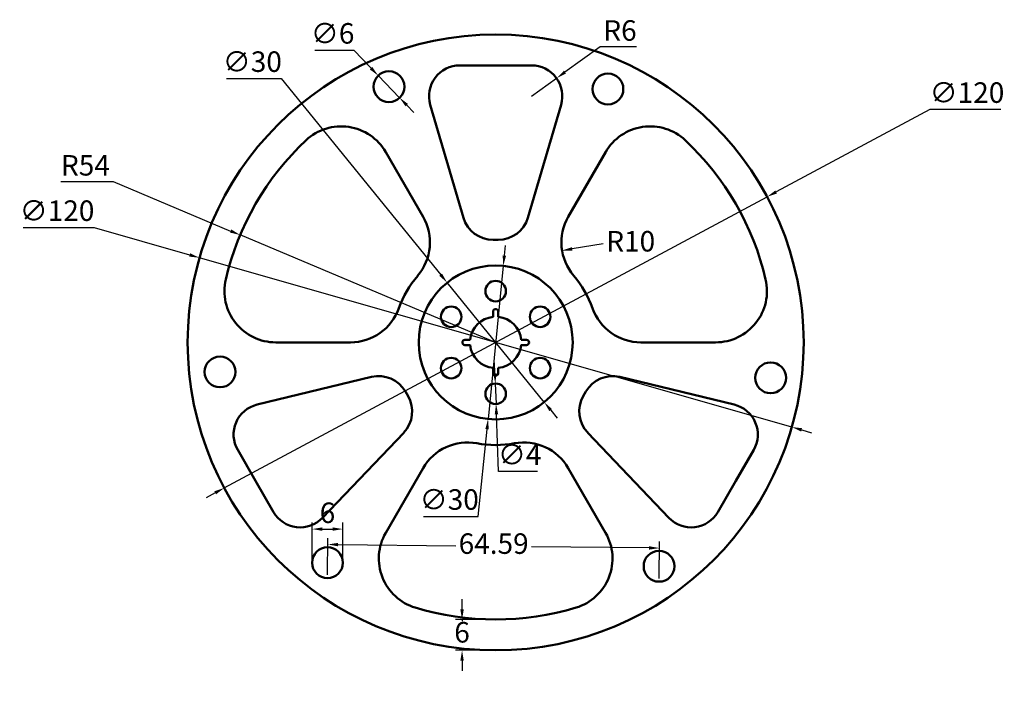
# Model space of a CAD drawing. Units: millimetres. Extents: x 45 to 237, y 22 to 152.
import ezdxf

# ---------------------------------------------------------------- set-up
doc = ezdxf.new("R2010")
doc.units = ezdxf.units.MM
doc.layers.add('M-DIMS', color=2, linetype='Continuous', lineweight=25)
doc.layers.add('M-OUTL', color=7, linetype='Continuous', lineweight=50)
doc.styles.get("Standard").update_dxf_attribs({"font": 'arial.ttf'})
doc.dimstyles.new('ISO-25', dxfattribs={"dimtxt": 4, "dimasz": 2, "dimexe": 1.25, "dimexo": 0.625, "dimtad": 1, "dimtih": 1, "dimtoh": 1, "dimtxsty": 'Standard', "dimcen": 2.5, "dimadec": 0, "dimazin": 0, "dimtfac": 1, "dimtmove": 0, "dimatfit": 3, "dimfxl": 1, "dimarcsym": 0})

# ---------------------------------------------------------------- blocks, each defined once
blk = doc.blocks.new('*U1')
for p, q in [((-0.5, 0.26), (-0.5, -0.76)), ((0.5, 0.26), (0.5, -0.76))]:
    blk.add_line(p, q)
blk.add_arc((0, 0.26), 0.5, 0, 180)
blk = doc.blocks.new('*U2')
at = {"layer": 'M-OUTL', "color": 0, "linetype": 'ByBlock', "lineweight": -2, "transparency": 16777216}
blk.add_blockref('*U1', (138.18, 94.73), dxfattribs=at)
for p, rotation in [((132.45, 88.99), 90), ((143.92, 88.99), 270), ((138.18, 83.26), 180)]:
    blk.add_blockref('*U1', p, dxfattribs=dict(at, rotation=rotation))
blk = doc.blocks.new('*U3')
blk.add_circle((0, 0), 2)
blk = doc.blocks.new('*U4')
at = {"layer": 'M-OUTL', "color": 0, "linetype": 'ByBlock', "lineweight": -2, "transparency": 16777216}
blk.add_blockref('*U3', (138.18, 98.99), dxfattribs=at)
for p, rotation in [((129.52, 93.99), 59.99999999999999), ((146.84, 93.99), 300), ((129.52, 83.99), 120), ((146.84, 83.99), 240), ((138.18, 78.99), 180)]:
    blk.add_blockref('*U3', p, dxfattribs=dict(at, rotation=rotation))
blk = doc.blocks.new('*U5')
for p, q in [((18.68, 3.44), (11.4, 16.05)), ((4.54, -21.05), (-10.02, -21.05))]:
    blk.add_line(p, q)
for centre, radius, start, end in [((2.74, 11.05), 10, 30, 133.1366), ((32.83, -21.05), 54, 133.1366, 166.8634), ((10.02, -1.56), 10, 319.4712, 30), ((-10.02, -11.05), 10, 166.8634, 270), ((32.83, -21.05), 20, 139.4712, 160.5288), ((4.54, -11.05), 10, 270, 340.5288)]:
    blk.add_arc(centre, radius, start, end)
blk = doc.blocks.new('*U6')
at = {"layer": 'M-OUTL', "color": 0, "linetype": 'ByBlock', "lineweight": -2, "transparency": 16777216}
for p, rotation in [((172.83, 106.9), 240), ((136.36, 50.04), 119.9999999999999)]:
    blk.add_blockref('*U5', p, dxfattribs=dict(at, rotation=rotation))
blk.add_blockref('*U5', (105.36, 110.05), dxfattribs=at)
blk = doc.blocks.new('*U7')
for p, q in [((0, 17), (-6.98, 17)), ((0, 17), (6.98, 17)), ((-6.27, -12.69), (-12.74, 9.31)), ((12.74, 9.31), (6.27, -12.69))]:
    blk.add_line(p, q)
for centre, start, end in [((-6.98, 11), 90, 196.3895), ((6.98, 11), 343.6105, 90), ((-0.51, -11), 196.3895, 270), ((0.51, -11), 270, 343.6105)]:
    blk.add_arc(centre, 6, start, end)
blk = doc.blocks.new('*U8')
at = {"layer": 'M-OUTL', "color": 0, "linetype": 'ByBlock', "lineweight": -2, "transparency": 16777216}
blk.add_blockref('*U7', (138.18, 125.99), dxfattribs=at)
for p, rotation in [((106.14, 70.49), 120), ((170.23, 70.49), 240)]:
    blk.add_blockref('*U7', p, dxfattribs=dict(at, rotation=rotation))
blk = doc.blocks.new('*U9')
blk.add_circle((0, 0), 3)
blk = doc.blocks.new('*U10')
at = {"layer": 'M-OUTL', "color": 0, "linetype": 'ByBlock', "lineweight": -2, "transparency": 16777216}
blk.add_blockref('*U9', (117.39, 138.83), dxfattribs=at)
for p, rotation in [((191.74, 82.09), 239.9999999999999), ((105.42, 46.07), 120)]:
    blk.add_blockref('*U9', p, dxfattribs=dict(at, rotation=rotation))
blk = doc.blocks.new('*U11')
blk.add_circle((0, 0), 3)
blk = doc.blocks.new('*U12')
at = {"layer": 'M-OUTL', "color": 0, "linetype": 'ByBlock', "lineweight": -2, "transparency": 16777216}
blk.add_blockref('*U11', (117.39, 138.83), dxfattribs=at)
for p, rotation in [((191.74, 82.09), 239.9999999999999), ((105.42, 46.07), 120)]:
    blk.add_blockref('*U11', p, dxfattribs=dict(at, rotation=rotation))
blk = doc.blocks.new('*D13')
at = {"layer": 'Defpoints', "color": 0, "transparency": 16777216}
for p in [(160.99, 108.49), (151.11, 106.9)]:
    blk.add_point(p, dxfattribs=at)
at = {"layer": 'M-DIMS', "color": 0, "lineweight": -2, "transparency": 16777216}
blk.add_line((159.09, 108.19), (153.09, 107.22), dxfattribs=at)
at = {"layer": 'M-DIMS', "color": 0, "transparency": 16777216}
blk.add_solid([(153.03, 107.55), (153.14, 106.89), (151.11, 106.9)], dxfattribs=at)
at = {"layer": 'M-DIMS', "color": 0, "transparency": 16777216, "insert": (164.49, 108.19), "char_height": 4, "attachment_point": 5}
blk.add_mtext('R10', dxfattribs=at)
blk = doc.blocks.new('*D14')
at = {"layer": 'Defpoints', "color": 0, "transparency": 16777216}
for p in [(150.04, 140.49), (145.16, 136.99)]:
    blk.add_point(p, dxfattribs=at)
at = {"layer": 'M-DIMS', "color": 0, "lineweight": -2, "transparency": 16777216}
for p, q in [((158.55, 146.59), (151.67, 141.66)), ((165.62, 146.59), (158.55, 146.59)), ((145.16, 136.99), (150.04, 140.49))]:
    blk.add_line(p, q, dxfattribs=at)
at = {"layer": 'M-DIMS', "color": 0, "transparency": 16777216}
blk.add_solid([(151.47, 141.93), (151.86, 141.39), (150.04, 140.49)], dxfattribs=at)
at = {"layer": 'M-DIMS', "color": 0, "transparency": 16777216, "insert": (162.4, 149.26), "char_height": 4, "attachment_point": 5}
blk.add_mtext('R6', dxfattribs=at)
blk = doc.blocks.new('*D15')
at = {"layer": 'Defpoints', "color": 0, "transparency": 16777216}
for p in [(115.3, 140.99), (119.47, 136.67)]:
    blk.add_point(p, dxfattribs=at)
at = {"layer": 'M-DIMS', "color": 0, "lineweight": -2, "transparency": 16777216}
for p, q in [((102.94, 145.92), (110.54, 145.92)), ((110.54, 145.92), (113.91, 142.42)), ((119.47, 136.67), (115.3, 140.99)), ((120.86, 135.23), (122.25, 133.8))]:
    blk.add_line(p, q, dxfattribs=at)
blk.add_arc((117.39, 138.83), 3, 101.9366, 157.9006, dxfattribs=at)
at = {"layer": 'M-DIMS', "color": 0, "transparency": 16777216}
for points in [[(114.15, 142.66), (113.67, 142.19), (115.3, 140.99)], [(121.1, 135.47), (120.62, 135), (119.47, 136.67)]]:
    blk.add_solid(points, dxfattribs=at)
at = {"layer": 'M-DIMS', "color": 0, "transparency": 16777216, "insert": (106.42, 148.7), "char_height": 4, "attachment_point": 5}
blk.add_mtext('∅6', dxfattribs=at)
blk = doc.blocks.new('*D16')
at = {"layer": 'Defpoints', "color": 0, "transparency": 16777216}
for p in [(88.41, 109.93), (138.18, 88.99)]:
    blk.add_point(p, dxfattribs=at)
at = {"layer": 'M-DIMS', "color": 0, "lineweight": -2, "transparency": 16777216}
for p, q in [((53.5, 120.33), (63.67, 120.33)), ((63.67, 120.33), (86.56, 110.7)), ((138.18, 88.99), (88.41, 109.93))]:
    blk.add_line(p, q, dxfattribs=at)
at = {"layer": 'M-DIMS', "color": 0, "transparency": 16777216}
blk.add_solid([(86.69, 111.01), (86.43, 110.4), (88.41, 109.93)], dxfattribs=at)
at = {"layer": 'M-DIMS', "color": 0, "transparency": 16777216, "insert": (58.27, 122.99), "char_height": 4, "attachment_point": 5}
blk.add_mtext('R54', dxfattribs=at)
blk = doc.blocks.new('*D17')
at = {"layer": 'Defpoints', "color": 0, "transparency": 16777216}
for p in [(80.5, 105.49), (195.87, 72.5)]:
    blk.add_point(p, dxfattribs=at)
at = {"layer": 'M-DIMS', "color": 0, "lineweight": -2, "transparency": 16777216}
for p, q in [((46.15, 111.37), (59.95, 111.37)), ((59.95, 111.37), (78.57, 106.04)), ((195.87, 72.5), (80.5, 105.49)), ((197.79, 71.95), (199.72, 71.4))]:
    blk.add_line(p, q, dxfattribs=at)
at = {"layer": 'M-DIMS', "color": 0, "transparency": 16777216}
for points in [[(78.66, 106.36), (78.48, 105.72), (80.5, 105.49)], [(197.89, 72.27), (197.7, 71.63), (195.87, 72.5)]]:
    blk.add_solid(points, dxfattribs=at)
at = {"layer": 'M-DIMS', "color": 0, "transparency": 16777216, "insert": (52.74, 114.15), "char_height": 4, "attachment_point": 5}
blk.add_mtext('∅120', dxfattribs=at)
blk = doc.blocks.new('*D18')
at = {"layer": 'Defpoints', "color": 0, "transparency": 16777216}
for p in [(138.11, 80.99), (138.26, 77)]:
    blk.add_point(p, dxfattribs=at)
at = {"layer": 'M-DIMS', "color": 0, "lineweight": -2, "transparency": 16777216}
for p, q in [((138.03, 82.99), (137.96, 84.99)), ((138.11, 80.99), (138.26, 77)), ((138.75, 63.84), (138.33, 75)), ((146.34, 63.84), (138.75, 63.84))]:
    blk.add_line(p, q, dxfattribs=at)
blk.add_arc((138.18, 78.99), 2, 236.3439, 1.5663, dxfattribs=at)
at = {"layer": 'M-DIMS', "color": 0, "transparency": 16777216}
for points in [[(138.37, 83), (137.7, 82.98), (138.11, 80.99)], [(138.67, 75.01), (138, 74.98), (138.26, 77)]]:
    blk.add_solid(points, dxfattribs=at)
at = {"layer": 'M-DIMS', "color": 0, "transparency": 16777216, "insert": (142.86, 66.62), "char_height": 4, "attachment_point": 5}
blk.add_mtext('∅4', dxfattribs=at)
blk = doc.blocks.new('*D19')
at = {"layer": 'Defpoints', "color": 0, "transparency": 16777216}
for p in [(128.73, 100.64), (147.64, 77.35)]:
    blk.add_point(p, dxfattribs=at)
at = {"layer": 'M-DIMS', "color": 0, "lineweight": -2, "transparency": 16777216}
for p, q in [((85.74, 140.41), (96.43, 140.41)), ((96.43, 140.41), (127.47, 102.19)), ((147.64, 77.35), (128.73, 100.64)), ((148.9, 75.8), (150.16, 74.25))]:
    blk.add_line(p, q, dxfattribs=at)
at = {"layer": 'M-DIMS', "color": 0, "transparency": 16777216}
for points in [[(127.73, 102.4), (127.21, 101.98), (128.73, 100.64)], [(149.16, 76.01), (148.64, 75.59), (147.64, 77.35)]]:
    blk.add_solid(points, dxfattribs=at)
at = {"layer": 'M-DIMS', "color": 0, "transparency": 16777216, "insert": (90.78, 143.19), "char_height": 4, "attachment_point": 5}
blk.add_mtext('∅30', dxfattribs=at)
blk = doc.blocks.new('*D20')
at = {"layer": 'Defpoints', "color": 0, "transparency": 16777216}
for p in [(139.67, 103.92), (136.7, 74.07)]:
    blk.add_point(p, dxfattribs=at)
at = {"layer": 'M-DIMS', "color": 0, "lineweight": -2, "transparency": 16777216}
for p, q in [((139.87, 105.91), (140.07, 107.9)), ((139.67, 103.92), (136.7, 74.07)), ((134.8, 55.08), (136.5, 72.08)), ((124.11, 55.08), (134.8, 55.08))]:
    blk.add_line(p, q, dxfattribs=at)
at = {"layer": 'M-DIMS', "color": 0, "transparency": 16777216}
for points in [[(139.54, 105.94), (140.2, 105.88), (139.67, 103.92)], [(136.17, 72.11), (136.83, 72.05), (136.7, 74.07)]]:
    blk.add_solid(points, dxfattribs=at)
at = {"layer": 'M-DIMS', "color": 0, "transparency": 16777216, "insert": (129.14, 57.86), "char_height": 4, "attachment_point": 5}
blk.add_mtext('∅30', dxfattribs=at)
blk = doc.blocks.new('*D21')
at = {"layer": 'Defpoints', "color": 0, "transparency": 16777216}
for p in [(108.42, 52.62), (102.42, 46.07), (108.42, 46.07)]:
    blk.add_point(p, dxfattribs=at)
at = {"layer": 'M-DIMS', "color": 0, "lineweight": -2, "transparency": 16777216}
for p, q in [((102.42, 46.69), (102.42, 53.87)), ((108.42, 46.69), (108.42, 53.87)), ((104.42, 52.62), (106.42, 52.62))]:
    blk.add_line(p, q, dxfattribs=at)
at = {"layer": 'M-DIMS', "color": 0, "transparency": 16777216}
for points in [[(104.42, 52.95), (104.42, 52.28), (102.42, 52.62)], [(106.42, 52.95), (106.42, 52.28), (108.42, 52.62)]]:
    blk.add_solid(points, dxfattribs=at)
at = {"layer": 'M-DIMS', "color": 0, "transparency": 16777216, "insert": (105.42, 55.28), "char_height": 4, "attachment_point": 5}
blk.add_mtext('6', dxfattribs=at)
blk = doc.blocks.new('*D22')
at = {"layer": 'Defpoints', "color": 0, "transparency": 16777216}
for p in [(131.63, 34.99), (138.18, 34.99), (138.18, 28.99)]:
    blk.add_point(p, dxfattribs=at)
at = {"layer": 'M-DIMS', "color": 0, "lineweight": -2, "transparency": 16777216}
for p, q in [((131.63, 36.99), (131.63, 38.99)), ((137.56, 34.99), (130.38, 34.99)), ((131.63, 34.99), (131.63, 34.66)), ((137.56, 28.99), (130.38, 28.99)), ((131.63, 28.99), (131.63, 29.33)), ((131.63, 26.99), (131.63, 24.99))]:
    blk.add_line(p, q, dxfattribs=at)
at = {"layer": 'M-DIMS', "color": 0, "transparency": 16777216}
for points in [[(131.3, 36.99), (131.97, 36.99), (131.63, 34.99)], [(131.3, 26.99), (131.97, 26.99), (131.63, 28.99)]]:
    blk.add_solid(points, dxfattribs=at)
at = {"layer": 'M-DIMS', "color": 0, "transparency": 16777216, "insert": (131.63, 31.99), "char_height": 4, "attachment_point": 5}
blk.add_mtext('6', dxfattribs=at)
blk = doc.blocks.new('*D23')
at = {"layer": 'Defpoints', "color": 0, "transparency": 16777216}
for p in [(170.08, 48.92), (105.42, 43.07), (170.01, 42.37)]:
    blk.add_point(p, dxfattribs=at)
at = {"layer": 'M-DIMS', "color": 0, "lineweight": -2, "transparency": 16777216}
for p, q in [((105.43, 43.69), (105.51, 50.87)), ((170.01, 42.99), (170.09, 50.17)), ((107.49, 49.59), (130.4, 49.35)), ((168.08, 48.94), (145.18, 49.19))]:
    blk.add_line(p, q, dxfattribs=at)
at = {"layer": 'M-DIMS', "color": 0, "transparency": 16777216}
for points in [[(107.5, 49.93), (107.49, 49.26), (105.5, 49.62)], [(168.08, 49.27), (168.07, 48.61), (170.08, 48.92)]]:
    blk.add_solid(points, dxfattribs=at)
at = {"layer": 'M-DIMS', "color": 0, "transparency": 16777216, "insert": (137.79, 49.27), "char_height": 4, "attachment_point": 5}
blk.add_mtext('64.59', dxfattribs=at)
blk = doc.blocks.new('*D24')
at = {"layer": 'Defpoints', "color": 0, "transparency": 16777216}
for p in [(191.05, 117.36), (85.31, 60.63)]:
    blk.add_point(p, dxfattribs=at)
at = {"layer": 'M-DIMS', "color": 0, "lineweight": -2, "transparency": 16777216}
for p, q in [((222.78, 134.38), (192.82, 118.31)), ((236.58, 134.38), (222.78, 134.38)), ((85.31, 60.63), (191.05, 117.36)), ((83.55, 59.68), (81.79, 58.74))]:
    blk.add_line(p, q, dxfattribs=at)
at = {"layer": 'M-DIMS', "color": 0, "transparency": 16777216}
for points in [[(192.66, 118.6), (192.97, 118.01), (191.05, 117.36)], [(83.39, 59.98), (83.71, 59.39), (85.31, 60.63)]]:
    blk.add_solid(points, dxfattribs=at)
at = {"layer": 'M-DIMS', "color": 0, "transparency": 16777216, "insert": (229.99, 137.16), "char_height": 4, "attachment_point": 5}
blk.add_mtext('∅120', dxfattribs=at)

msp = doc.modelspace()

# ---------------------------------------------------------------- linework, layer by layer
at = {"layer": 'M-OUTL'}
for p, q in [((138.183, 108.995), (137.673, 108.995)), ((138.183, 108.995), (138.694, 108.995)), ((120.608, 79.437), (121.118, 78.552)), ((155.249, 78.552), (155.759, 79.437))]:
    msp.add_line(p, q, dxfattribs=at)
for radius in [60, 15]:
    msp.add_circle((138.183, 88.995), radius, dxfattribs=at)
for start, end in [(95.73917, 174.26083), (5.73917, 84.26083), (185.73917, 264.26083), (275.73917, 354.26083)]:
    msp.add_arc((138.183, 88.995), 5, start, end, dxfattribs=at)

# ---------------------------------------------------------------- block references
at = {"layer": 'M-OUTL', "xscale": -1, "rotation": 358.7627453625808}
msp.add_blockref('*U12', (274.413, -2.963), dxfattribs=at)
at = {"layer": 'M-OUTL'}
for name in ['*U8', '*U10', '*U6', '*U4', '*U2']:
    msp.add_blockref(name, (0, 0), dxfattribs=at)

# ---------------------------------------------------------------- dimensions: what is measured, and where the dimension line sits
at = {"layer": 'M-DIMS'}
for center, mpoint, picture, middle in [((145.164, 136.995), (150.041, 140.491), '*D14', (162.401, 146.594)), ((138.183, 88.995), (88.406, 109.928), '*D16', (58.273, 120.33)), ((160.986, 108.49), (151.112, 106.903), '*D13', (159.095, 108.186))]:
    dim = msp.add_radius_dim(center=center, mpoint=mpoint, dimstyle='ISO-25', override={"dimclrd": 0, "dimclre": 0, "dimclrt": 0}, dxfattribs=at)
    dim.commit()
    dim.dimension.update_dxf_attribs({"geometry": picture, "text_midpoint": middle, "dimtype": 164})
for p1, p2, override, picture, middle in [((119.471, 136.672), (115.301, 140.986), {"dimclrd": 0, "dimclre": 0, "dimclrt": 0}, '*D15', (106.425, 145.916)), ((147.639, 77.35), (128.728, 100.639), {"dimclrd": 0, "dimclre": 0, "dimclrt": 0}, '*D19', (90.775, 140.407)), ((85.313, 60.627), (191.054, 117.362), {"dimdec": 0, "dimlfac": 1, "dimrnd": 0, "dimzin": 0, "dimdsep": 46, "dimlunit": 2}, '*D24', (229.989, 134.382)), ((195.871, 72.498), (80.496, 105.491), {"dimclrd": 0, "dimclre": 0, "dimclrt": 0}, '*D17', (52.736, 111.367)), ((139.671, 103.921), (136.696, 74.069), {"dimclrd": 0, "dimclre": 0, "dimclrt": 0}, '*D20', (129.144, 55.082)), ((138.108, 80.993), (138.258, 76.996), {"dimclrd": 0, "dimclre": 0, "dimclrt": 0}, '*D18', (142.857, 63.836))]:
    dim = msp.add_diameter_dim_2p(p1=p1, p2=p2, dimstyle='ISO-25', override=override, dxfattribs=at)
    dim.commit()
    dim.dimension.update_dxf_attribs({"geometry": picture, "text_midpoint": middle, "dimtype": 163})
dim = msp.add_linear_dim(base=(108.424, 52.616), p1=(102.424, 46.066), p2=(108.424, 46.066), dimstyle='ISO-25', override={"dimdec": 0, "dimlfac": 1, "dimrnd": 0, "dimzin": 0, "dimdsep": 46, "dimlunit": 2}, dxfattribs=at)
dim.commit()
dim.dimension.update_dxf_attribs({"geometry": '*D21', "text_midpoint": (105.424, 55.284)})
for base, p1, p2, angle, override, picture, middle in [((170.078, 48.918), (105.424, 43.066), (170.008, 42.369), 359.38137, {"dimdec": 2, "dimlfac": 1, "dimrnd": 0, "dimzin": 0, "dimdsep": 46, "dimlunit": 2}, '*D23', (137.787, 49.267)), ((131.633, 34.995), (138.183, 28.995), (138.183, 34.995), 90, {"dimdec": 0, "dimlfac": 1, "dimrnd": 0, "dimzin": 0, "dimdsep": 46, "dimlunit": 2}, '*D22', (131.633, 31.995))]:
    dim = msp.add_linear_dim(base=base, p1=p1, p2=p2, angle=angle, dimstyle='ISO-25', override=override, dxfattribs=at)
    dim.commit()
    dim.dimension.update_dxf_attribs({"geometry": picture, "text_midpoint": middle})

doc.saveas('drawing.dxf')
